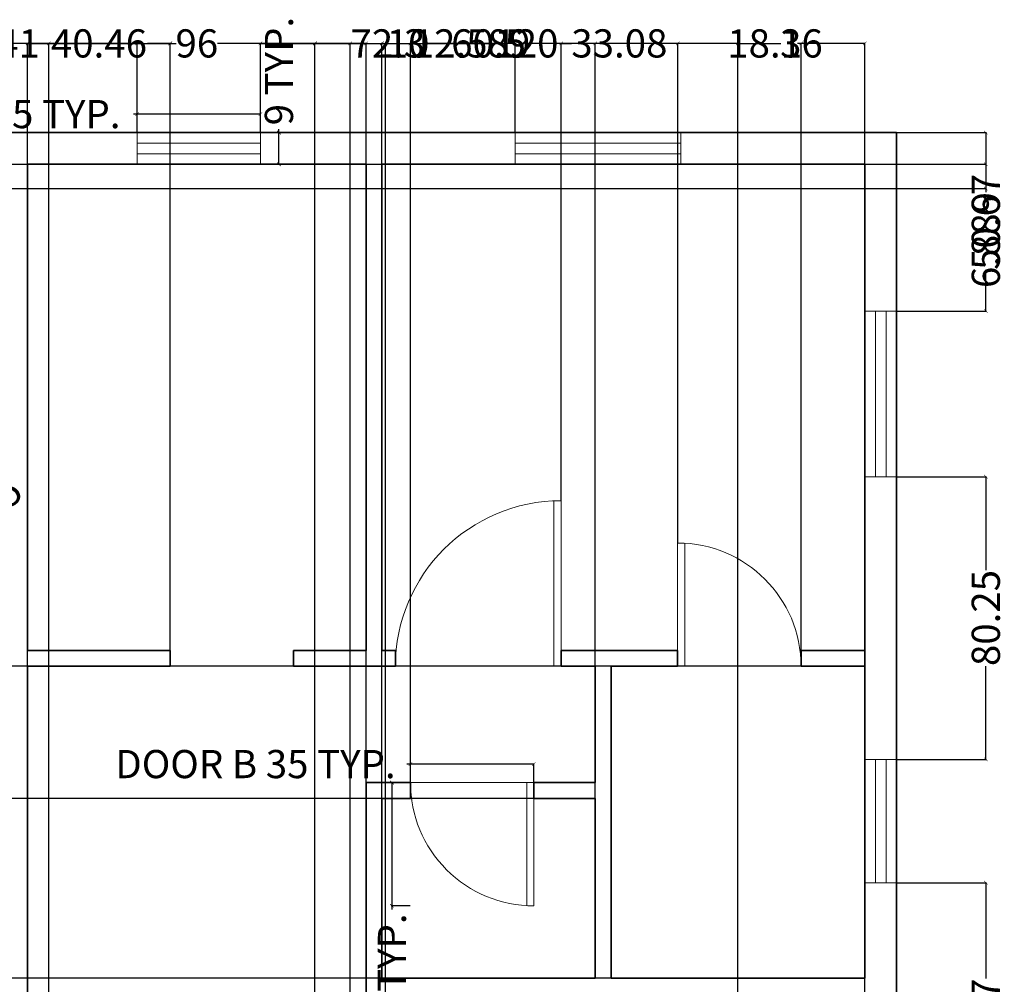
# Model space of a CAD drawing. Units: inches. Extents: x 878 to 1443, y 634 to 1188.
# Tile 5 of 5: x 1164 to 1443, y 879 to 1153. Entities that reach past the tile are written whole.
import ezdxf

# ---------------------------------------------------------------- set-up
doc = ezdxf.new("R2010")
doc.units = ezdxf.units.IN
doc.header["$MEASUREMENT"] = 0
doc.layers.add('A-ANNO-DIMS', color=2, linetype='Continuous', lineweight=18)
doc.layers.add('A-WALL', color=7, linetype='Continuous', lineweight=35)
doc.layers.add('A-DOOR', color=41, linetype='Continuous', lineweight=18, true_color=0xf4ee51)
doc.layers.add('A-GLAZ', color=152, linetype='Continuous', lineweight=18, true_color=0x2776bb)
doc.styles.get("Standard").update_dxf_attribs({"font": 'arial.ttf'})
doc.dimstyles.get("Standard").update_dxf_attribs({"dimtxt": 8, "dimasz": 1, "dimexe": 0.18, "dimexo": 0.0625, "dimgap": 0.09, "dimtad": 0, "dimdec": 4, "dimzin": 0, "dimdsep": 46, "dimlunit": 3, "dimtxsty": 'Standard', "dimblk": 'ARCHTICK', "dimcen": 0.09, "dimclrd": 6, "dimclre": 5, "dimclrt": 140, "dimadec": 0, "dimazin": 0, "dimtfac": 1, "dimtdec": 4, "dimtofl": 0, "dimtmove": 0, "dimatfit": 3, "dimfxl": 1, "dimtolj": 1, "dimtzin": 0, "dimarcsym": 0})

# ---------------------------------------------------------------- blocks, each defined once
blk = doc.blocks.new('WIN-47IN')
for p, q in [((9, 47), (0, 47)), ((0, 47), (0, 0)), ((3, 0), (3, 47)), ((6, 0), (6, 47)), ((9, 0), (9, 47)), ((0, 0), (9, 0))]:
    blk.add_line(p, q)
blk = doc.blocks.new('WIN-35IN')
for p, q in [((0, 35), (0, 0)), ((9, 35), (0, 35)), ((3, 0), (3, 35)), ((6, 0), (6, 35)), ((9, 0), (9, 35)), ((0, 0), (9, 0))]:
    blk.add_line(p, q)
blk = doc.blocks.new('DOOR-47IN')
for p, q in [((0, 47), (0, 0)), ((0, 2), (46.96, 2)), ((0, 0), (47, 0))]:
    blk.add_line(p, q)
blk.add_arc((0, 0), 47, 0, 90)
blk = doc.blocks.new('DOOR-35IN')
for p, q in [((0, 35), (0, 0)), ((2, 34.94), (2, 0)), ((0, 0), (35, 0))]:
    blk.add_line(p, q)
blk.add_arc((0, 0), 35, 360, 90)
blk = doc.blocks.new('_ArchTick')
at = {"color": 0, "linetype": 'ByBlock', "const_width": 0.15}
blk.add_lwpolyline([(-0.5, -0.5), (0.5, 0.5)], dxfattribs=at)
blk = doc.blocks.new('*D11')
at = {"layer": 'A-ANNO-DIMS', "color": 6, "lineweight": -2, "transparency": 16777216}
for p, q in [((1197.44, 1125.72), (1196.44, 1125.72)), ((1232.44, 1125.72), (1197.44, 1125.72))]:
    blk.add_line(p, q, dxfattribs=at)
at = {"layer": 'A-ANNO-DIMS', "color": 5, "lineweight": -2, "transparency": 16777216}
for p, q in [((1197.44, 1120.53), (1197.44, 1125.9)), ((1232.44, 1120.53), (1232.44, 1125.9))]:
    blk.add_line(p, q, dxfattribs=at)
at = {"layer": 'Defpoints', "color": 0, "lineweight": -2, "transparency": 16777216}
for p in [(1197.44, 1125.72), (1197.44, 1120.47), (1232.44, 1120.47)]:
    blk.add_point(p, dxfattribs=at)
at = {"layer": 'A-ANNO-DIMS', "color": 6, "lineweight": -2, "transparency": 16777216}
for p, rotation in [((1197.44, 1125.72), 179.9999999999992), ((1232.44, 1125.72), 359.9999999999992)]:
    blk.add_blockref('_ArchTick', p, dxfattribs=dict(at, rotation=rotation))
at = {"layer": 'A-ANNO-DIMS', "color": 140, "transparency": 16777216, "insert": (1145.37, 1125.72), "char_height": 8, "attachment_point": 5}
blk.add_mtext('\\A1;WINDOW B 35 TYP.', dxfattribs=at)
blk = doc.blocks.new('*D12')
at = {"layer": 'A-ANNO-DIMS', "color": 5, "lineweight": -2, "transparency": 16777216}
for p, q in [((1232.5, 1120.47), (1237.87, 1120.47)), ((1232.5, 1111.47), (1237.87, 1111.47))]:
    blk.add_line(p, q, dxfattribs=at)
at = {"layer": 'A-ANNO-DIMS', "color": 6, "lineweight": -2, "transparency": 16777216}
for p, q in [((1237.69, 1120.47), (1237.69, 1121.47)), ((1237.69, 1111.47), (1237.69, 1120.47))]:
    blk.add_line(p, q, dxfattribs=at)
at = {"layer": 'Defpoints', "color": 0, "lineweight": -2, "transparency": 16777216}
for p in [(1232.44, 1120.47), (1237.69, 1120.47), (1232.44, 1111.47)]:
    blk.add_point(p, dxfattribs=at)
at = {"layer": 'A-ANNO-DIMS', "color": 6, "lineweight": -2, "transparency": 16777216}
for p, rotation in [((1237.69, 1120.47), 90), ((1237.69, 1111.47), 270)]:
    blk.add_blockref('_ArchTick', p, dxfattribs=dict(at, rotation=rotation))
at = {"layer": 'A-ANNO-DIMS', "color": 140, "transparency": 16777216, "insert": (1237.69, 1137.92), "char_height": 8, "attachment_point": 5, "rotation": 90}
blk.add_mtext('\\A1;9 TYP.', dxfattribs=at)
blk = doc.blocks.new('*D17')
at = {"layer": 'A-ANNO-DIMS', "color": 5, "lineweight": -2, "transparency": 16777216}
for p, q in [((1274.99, 936.03), (1274.99, 941.4)), ((1309.99, 936.03), (1309.99, 941.4))]:
    blk.add_line(p, q, dxfattribs=at)
at = {"layer": 'A-ANNO-DIMS', "color": 6, "lineweight": -2, "transparency": 16777216}
for p, q in [((1274.99, 941.22), (1273.99, 941.22)), ((1309.99, 941.22), (1274.99, 941.22))]:
    blk.add_line(p, q, dxfattribs=at)
at = {"layer": 'Defpoints', "color": 0, "lineweight": -2, "transparency": 16777216}
for p in [(1274.99, 941.22), (1274.99, 935.97), (1309.99, 935.97)]:
    blk.add_point(p, dxfattribs=at)
at = {"layer": 'A-ANNO-DIMS', "color": 6, "lineweight": -2, "transparency": 16777216, "rotation": 180}
blk.add_blockref('_ArchTick', (1274.99, 941.22), dxfattribs=at)
at = {"layer": 'A-ANNO-DIMS', "color": 6, "lineweight": -2, "transparency": 16777216}
blk.add_blockref('_ArchTick', (1309.99, 941.22), dxfattribs=at)
at = {"layer": 'A-ANNO-DIMS', "color": 140, "transparency": 16777216, "insert": (1231.03, 941.22), "char_height": 8, "attachment_point": 5}
blk.add_mtext('\\A1;DOOR B 35 TYP.', dxfattribs=at)
blk = doc.blocks.new('*D18')
at = {"layer": 'A-ANNO-DIMS', "color": 5, "lineweight": -2, "transparency": 16777216}
for p, q in [((1274.92, 935.97), (1269.56, 935.97)), ((1274.92, 900.97), (1269.56, 900.97))]:
    blk.add_line(p, q, dxfattribs=at)
at = {"layer": 'A-ANNO-DIMS', "color": 6, "lineweight": -2, "transparency": 16777216}
for p, q in [((1269.74, 935.97), (1269.74, 900.97)), ((1269.74, 900.97), (1269.74, 899.97))]:
    blk.add_line(p, q, dxfattribs=at)
at = {"layer": 'Defpoints', "color": 0, "lineweight": -2, "transparency": 16777216}
for p in [(1274.99, 935.97), (1269.74, 900.97), (1274.99, 900.97)]:
    blk.add_point(p, dxfattribs=at)
at = {"layer": 'A-ANNO-DIMS', "color": 6, "lineweight": -2, "transparency": 16777216}
for p, rotation in [((1269.74, 935.97), 90), ((1269.74, 900.97), 270)]:
    blk.add_blockref('_ArchTick', p, dxfattribs=dict(at, rotation=rotation))
at = {"layer": 'A-ANNO-DIMS', "color": 140, "transparency": 16777216, "insert": (1269.74, 880.41), "char_height": 8, "attachment_point": 5, "rotation": 90}
blk.add_mtext('\\A1;35 TYP.', dxfattribs=at)
blk = doc.blocks.new('*D26')
at = {"layer": 'A-ANNO-DIMS', "color": 5, "lineweight": -2, "transparency": 16777216}
for p, q in [((1115.03, 1120.53), (1115.03, 1145.96)), ((1197.44, 1120.53), (1197.44, 1145.96))]:
    blk.add_line(p, q, dxfattribs=at)
at = {"layer": 'A-ANNO-DIMS', "color": 6, "lineweight": -2, "transparency": 16777216}
for p, q in [((1115.03, 1145.78), (1143.42, 1145.78)), ((1197.44, 1145.78), (1169.06, 1145.78))]:
    blk.add_line(p, q, dxfattribs=at)
at = {"layer": 'Defpoints', "color": 0, "lineweight": -2, "transparency": 16777216}
for p in [(1197.44, 1145.78), (1115.03, 1120.47), (1197.44, 1120.47)]:
    blk.add_point(p, dxfattribs=at)
at = {"layer": 'A-ANNO-DIMS', "color": 6, "lineweight": -2, "transparency": 16777216, "rotation": 180}
blk.add_blockref('_ArchTick', (1115.03, 1145.78), dxfattribs=at)
at = {"layer": 'A-ANNO-DIMS', "color": 6, "lineweight": -2, "transparency": 16777216}
blk.add_blockref('_ArchTick', (1197.44, 1145.78), dxfattribs=at)
at = {"layer": 'A-ANNO-DIMS', "color": 140, "transparency": 16777216, "insert": (1156.24, 1145.78), "char_height": 8, "attachment_point": 5}
blk.add_mtext('\\A1;82.41', dxfattribs=at)
blk = doc.blocks.new('*D27')
at = {"layer": 'A-ANNO-DIMS', "color": 5, "lineweight": -2, "transparency": 16777216}
for p, q in [((1232.44, 1120.53), (1232.44, 1145.96)), ((1304.74, 1120.53), (1304.74, 1145.96))]:
    blk.add_line(p, q, dxfattribs=at)
at = {"layer": 'A-ANNO-DIMS', "color": 6, "lineweight": -2, "transparency": 16777216}
for p, q in [((1232.44, 1145.78), (1258.14, 1145.78)), ((1304.74, 1145.78), (1279.04, 1145.78))]:
    blk.add_line(p, q, dxfattribs=at)
at = {"layer": 'Defpoints', "color": 0, "lineweight": -2, "transparency": 16777216}
for p in [(1304.74, 1145.78), (1232.44, 1120.47), (1304.74, 1120.47)]:
    blk.add_point(p, dxfattribs=at)
at = {"layer": 'A-ANNO-DIMS', "color": 6, "lineweight": -2, "transparency": 16777216, "rotation": 180}
blk.add_blockref('_ArchTick', (1232.44, 1145.78), dxfattribs=at)
at = {"layer": 'A-ANNO-DIMS', "color": 6, "lineweight": -2, "transparency": 16777216}
blk.add_blockref('_ArchTick', (1304.74, 1145.78), dxfattribs=at)
at = {"layer": 'A-ANNO-DIMS', "color": 140, "transparency": 16777216, "insert": (1268.59, 1145.78), "char_height": 8, "attachment_point": 5}
blk.add_mtext('\\A1;72.3', dxfattribs=at)
blk = doc.blocks.new('*D30')
at = {"layer": 'A-ANNO-DIMS', "color": 5, "lineweight": -2, "transparency": 16777216}
for p, q in [((1412.96, 1120.47), (1438.39, 1120.47)), ((1412.96, 1069.8), (1438.39, 1069.8))]:
    blk.add_line(p, q, dxfattribs=at)
at = {"layer": 'A-ANNO-DIMS', "color": 6, "lineweight": -2, "transparency": 16777216}
for p, q in [((1438.21, 1120.47), (1438.21, 1108.72)), ((1438.21, 1069.8), (1438.21, 1081.55))]:
    blk.add_line(p, q, dxfattribs=at)
at = {"layer": 'Defpoints', "color": 0, "lineweight": -2, "transparency": 16777216}
for p in [(1412.9, 1120.47), (1412.9, 1069.8), (1438.21, 1069.8)]:
    blk.add_point(p, dxfattribs=at)
at = {"layer": 'A-ANNO-DIMS', "color": 6, "lineweight": -2, "transparency": 16777216}
for p, rotation in [((1438.21, 1120.47), 90), ((1438.21, 1069.8), 270)]:
    blk.add_blockref('_ArchTick', p, dxfattribs=dict(at, rotation=rotation))
at = {"layer": 'A-ANNO-DIMS', "color": 140, "transparency": 16777216, "insert": (1438.21, 1095.14), "char_height": 8, "attachment_point": 5, "rotation": 90}
blk.add_mtext('\\A1;50.67', dxfattribs=at)
blk = doc.blocks.new('*D31')
at = {"layer": 'A-ANNO-DIMS', "color": 5, "lineweight": -2, "transparency": 16777216}
for p, q in [((1412.96, 1022.8), (1438.39, 1022.8)), ((1412.96, 942.55), (1438.39, 942.55))]:
    blk.add_line(p, q, dxfattribs=at)
at = {"layer": 'A-ANNO-DIMS', "color": 6, "lineweight": -2, "transparency": 16777216}
for p, q in [((1438.21, 1022.8), (1438.21, 996.3)), ((1438.21, 942.55), (1438.21, 969.05))]:
    blk.add_line(p, q, dxfattribs=at)
at = {"layer": 'Defpoints', "color": 0, "lineweight": -2, "transparency": 16777216}
for p in [(1412.9, 1022.8), (1412.9, 942.55), (1438.21, 942.55)]:
    blk.add_point(p, dxfattribs=at)
at = {"layer": 'A-ANNO-DIMS', "color": 6, "lineweight": -2, "transparency": 16777216}
for p, rotation in [((1438.21, 1022.8), 90), ((1438.21, 942.55), 270)]:
    blk.add_blockref('_ArchTick', p, dxfattribs=dict(at, rotation=rotation))
at = {"layer": 'A-ANNO-DIMS', "color": 140, "transparency": 16777216, "insert": (1438.21, 982.68), "char_height": 8, "attachment_point": 5, "rotation": 90}
blk.add_mtext('\\A1;80.25', dxfattribs=at)
blk = doc.blocks.new('*D32')
at = {"layer": 'A-ANNO-DIMS', "color": 5, "lineweight": -2, "transparency": 16777216}
for p, q in [((1412.96, 907.55), (1438.39, 907.55)), ((1412.96, 825.89), (1438.39, 825.89))]:
    blk.add_line(p, q, dxfattribs=at)
at = {"layer": 'A-ANNO-DIMS', "color": 6, "lineweight": -2, "transparency": 16777216}
for p, q in [((1438.21, 907.55), (1438.21, 880.32)), ((1438.21, 825.89), (1438.21, 853.13))]:
    blk.add_line(p, q, dxfattribs=at)
at = {"layer": 'Defpoints', "color": 0, "lineweight": -2, "transparency": 16777216}
for p in [(1412.9, 907.55), (1412.9, 825.89), (1438.21, 825.89)]:
    blk.add_point(p, dxfattribs=at)
at = {"layer": 'A-ANNO-DIMS', "color": 6, "lineweight": -2, "transparency": 16777216}
for p, rotation in [((1438.21, 907.55), 90), ((1438.21, 825.89), 270)]:
    blk.add_blockref('_ArchTick', p, dxfattribs=dict(at, rotation=rotation))
at = {"layer": 'A-ANNO-DIMS', "color": 140, "transparency": 16777216, "insert": (1438.21, 866.72), "char_height": 8, "attachment_point": 5, "rotation": 90}
blk.add_mtext('\\A1;81.67', dxfattribs=at)
blk = doc.blocks.new('*D35')
at = {"layer": 'A-ANNO-DIMS', "color": 5, "lineweight": -2, "transparency": 16777216}
for p, q in [((1166.4, 760.53), (1166.4, 1145.96)), ((1262.4, 760.53), (1262.4, 1145.96))]:
    blk.add_line(p, q, dxfattribs=at)
at = {"layer": 'A-ANNO-DIMS', "color": 6, "lineweight": -2, "transparency": 16777216}
for p, q in [((1166.4, 1145.78), (1208.58, 1145.78)), ((1262.4, 1145.78), (1220.22, 1145.78))]:
    blk.add_line(p, q, dxfattribs=at)
at = {"layer": 'Defpoints', "color": 0, "lineweight": -2, "transparency": 16777216}
for p in [(1262.4, 1145.78), (1166.4, 760.47), (1262.4, 760.47)]:
    blk.add_point(p, dxfattribs=at)
at = {"layer": 'A-ANNO-DIMS', "color": 6, "lineweight": -2, "transparency": 16777216, "rotation": 180}
blk.add_blockref('_ArchTick', (1166.4, 1145.78), dxfattribs=at)
at = {"layer": 'A-ANNO-DIMS', "color": 6, "lineweight": -2, "transparency": 16777216}
blk.add_blockref('_ArchTick', (1262.4, 1145.78), dxfattribs=at)
at = {"layer": 'A-ANNO-DIMS', "color": 140, "transparency": 16777216, "insert": (1214.4, 1145.78), "char_height": 8, "attachment_point": 5}
blk.add_mtext('\\A1;96', dxfattribs=at)
blk = doc.blocks.new('*D37')
at = {"layer": 'A-ANNO-DIMS', "color": 5, "lineweight": -2, "transparency": 16777216}
for p, q in [((1403.84, 968.97), (883.41, 968.97)), ((1403.84, 880.47), (883.41, 880.47))]:
    blk.add_line(p, q, dxfattribs=at)
at = {"layer": 'A-ANNO-DIMS', "color": 6, "lineweight": -2, "transparency": 16777216}
for p, q in [((883.59, 968.97), (883.59, 935.24)), ((883.59, 880.47), (883.59, 914.2))]:
    blk.add_line(p, q, dxfattribs=at)
at = {"layer": 'Defpoints', "color": 0, "lineweight": -2, "transparency": 16777216}
for p in [(1403.9, 968.97), (883.59, 880.47), (1403.9, 880.47)]:
    blk.add_point(p, dxfattribs=at)
at = {"layer": 'A-ANNO-DIMS', "color": 6, "lineweight": -2, "transparency": 16777216}
for p, rotation in [((883.59, 968.97), 90), ((883.59, 880.47), 270)]:
    blk.add_blockref('_ArchTick', p, dxfattribs=dict(at, rotation=rotation))
at = {"layer": 'A-ANNO-DIMS', "color": 140, "transparency": 16777216, "insert": (883.59, 924.72), "char_height": 8, "attachment_point": 5, "rotation": 90}
blk.add_mtext('\\A1;88.5', dxfattribs=at)
blk = doc.blocks.new('*D41')
at = {"layer": 'A-ANNO-DIMS', "color": 5, "lineweight": -2, "transparency": 16777216}
for p, q in [((1266.9, 880.53), (1266.9, 1145.96)), ((1327.4, 880.53), (1327.4, 1145.96))]:
    blk.add_line(p, q, dxfattribs=at)
at = {"layer": 'A-ANNO-DIMS', "color": 6, "lineweight": -2, "transparency": 16777216}
for p, q in [((1266.9, 1145.78), (1286.62, 1145.78)), ((1327.4, 1145.78), (1307.68, 1145.78))]:
    blk.add_line(p, q, dxfattribs=at)
at = {"layer": 'Defpoints', "color": 0, "lineweight": -2, "transparency": 16777216}
for p in [(1327.4, 1145.78), (1266.9, 880.47), (1327.4, 880.47)]:
    blk.add_point(p, dxfattribs=at)
at = {"layer": 'A-ANNO-DIMS', "color": 6, "lineweight": -2, "transparency": 16777216, "rotation": 180}
blk.add_blockref('_ArchTick', (1266.9, 1145.78), dxfattribs=at)
at = {"layer": 'A-ANNO-DIMS', "color": 6, "lineweight": -2, "transparency": 16777216}
blk.add_blockref('_ArchTick', (1327.4, 1145.78), dxfattribs=at)
at = {"layer": 'A-ANNO-DIMS', "color": 140, "transparency": 16777216, "insert": (1297.15, 1145.78), "char_height": 8, "attachment_point": 5}
blk.add_mtext('\\A1;60.5', dxfattribs=at)
blk = doc.blocks.new('*D43')
at = {"layer": 'A-ANNO-DIMS', "color": 5, "lineweight": -2, "transparency": 16777216}
for p, q in [((1327.34, 931.47), (883.41, 931.47)), ((1327.34, 880.47), (883.41, 880.47))]:
    blk.add_line(p, q, dxfattribs=at)
at = {"layer": 'A-ANNO-DIMS', "color": 6, "lineweight": -2, "transparency": 16777216}
for p, q in [((883.59, 931.47), (883.59, 911.02)), ((883.59, 880.47), (883.59, 900.92))]:
    blk.add_line(p, q, dxfattribs=at)
at = {"layer": 'Defpoints', "color": 0, "lineweight": -2, "transparency": 16777216}
for p in [(883.59, 931.47), (1327.4, 931.47), (1327.4, 880.47)]:
    blk.add_point(p, dxfattribs=at)
at = {"layer": 'A-ANNO-DIMS', "color": 6, "lineweight": -2, "transparency": 16777216}
for p, rotation in [((883.59, 931.47), 90), ((883.59, 880.47), 270)]:
    blk.add_blockref('_ArchTick', p, dxfattribs=dict(at, rotation=rotation))
at = {"layer": 'A-ANNO-DIMS', "color": 140, "transparency": 16777216, "insert": (883.59, 905.97), "char_height": 8, "attachment_point": 5, "rotation": 90}
blk.add_mtext('\\A1;51', dxfattribs=at)
blk = doc.blocks.new('*D46')
at = {"layer": 'A-ANNO-DIMS', "color": 5, "lineweight": -2, "transparency": 16777216}
for p, q in [((1110.3, 751.53), (1110.3, 1145.96)), ((1172.39, 751.53), (1172.39, 1145.96))]:
    blk.add_line(p, q, dxfattribs=at)
at = {"layer": 'A-ANNO-DIMS', "color": 6, "lineweight": -2, "transparency": 16777216}
for p, q in [((1110.3, 1145.78), (1127.73, 1145.78)), ((1172.39, 1145.78), (1154.96, 1145.78))]:
    blk.add_line(p, q, dxfattribs=at)
at = {"layer": 'Defpoints', "color": 0, "lineweight": -2, "transparency": 16777216}
for p in [(1172.39, 1145.78), (1110.3, 751.47), (1172.39, 751.47)]:
    blk.add_point(p, dxfattribs=at)
at = {"layer": 'A-ANNO-DIMS', "color": 6, "lineweight": -2, "transparency": 16777216, "rotation": 180}
blk.add_blockref('_ArchTick', (1110.3, 1145.78), dxfattribs=at)
at = {"layer": 'A-ANNO-DIMS', "color": 6, "lineweight": -2, "transparency": 16777216}
blk.add_blockref('_ArchTick', (1172.39, 1145.78), dxfattribs=at)
at = {"layer": 'A-ANNO-DIMS', "color": 140, "transparency": 16777216, "insert": (1141.35, 1145.78), "char_height": 8, "attachment_point": 5}
blk.add_mtext('\\A1;62.08', dxfattribs=at)
blk = doc.blocks.new('*D51')
at = {"layer": 'A-ANNO-DIMS', "color": 5, "lineweight": -2, "transparency": 16777216}
for p, q in [((1166.4, 973.53), (1166.4, 1145.96)), ((1206.86, 973.53), (1206.86, 1145.96))]:
    blk.add_line(p, q, dxfattribs=at)
at = {"layer": 'A-ANNO-DIMS', "color": 6, "lineweight": -2, "transparency": 16777216}
for p, q in [((1166.4, 1145.78), (1172.88, 1145.78)), ((1206.86, 1145.78), (1200.37, 1145.78))]:
    blk.add_line(p, q, dxfattribs=at)
at = {"layer": 'Defpoints', "color": 0, "lineweight": -2, "transparency": 16777216}
for p in [(1206.86, 1145.78), (1166.4, 973.47), (1206.86, 973.47)]:
    blk.add_point(p, dxfattribs=at)
at = {"layer": 'A-ANNO-DIMS', "color": 6, "lineweight": -2, "transparency": 16777216, "rotation": 180}
blk.add_blockref('_ArchTick', (1166.4, 1145.78), dxfattribs=at)
at = {"layer": 'A-ANNO-DIMS', "color": 6, "lineweight": -2, "transparency": 16777216}
blk.add_blockref('_ArchTick', (1206.86, 1145.78), dxfattribs=at)
at = {"layer": 'A-ANNO-DIMS', "color": 140, "transparency": 16777216, "insert": (1186.63, 1145.78), "char_height": 8, "attachment_point": 5}
blk.add_mtext('\\A1;40.46', dxfattribs=at)
blk = doc.blocks.new('*D54')
at = {"layer": 'A-ANNO-DIMS', "color": 6, "lineweight": -2, "transparency": 16777216}
for p, q in [((1385.8, 1145.78), (1384.8, 1145.78)), ((1403.9, 1145.78), (1385.8, 1145.78))]:
    blk.add_line(p, q, dxfattribs=at)
at = {"layer": 'A-ANNO-DIMS', "color": 5, "lineweight": -2, "transparency": 16777216}
for p, q in [((1385.8, 973.53), (1385.8, 1145.96)), ((1403.9, 973.53), (1403.9, 1145.96))]:
    blk.add_line(p, q, dxfattribs=at)
at = {"layer": 'Defpoints', "color": 0, "lineweight": -2, "transparency": 16777216}
for p in [(1385.8, 1145.78), (1385.8, 973.47), (1403.9, 973.47)]:
    blk.add_point(p, dxfattribs=at)
at = {"layer": 'A-ANNO-DIMS', "color": 6, "lineweight": -2, "transparency": 16777216, "rotation": 180}
blk.add_blockref('_ArchTick', (1385.8, 1145.78), dxfattribs=at)
at = {"layer": 'A-ANNO-DIMS', "color": 6, "lineweight": -2, "transparency": 16777216}
blk.add_blockref('_ArchTick', (1403.9, 1145.78), dxfattribs=at)
at = {"layer": 'A-ANNO-DIMS', "color": 140, "transparency": 16777216, "insert": (1375.47, 1145.78), "char_height": 8, "attachment_point": 5}
blk.add_mtext('\\A1;18.1', dxfattribs=at)
blk = doc.blocks.new('*D55')
at = {"layer": 'A-ANNO-DIMS', "color": 5, "lineweight": -2, "transparency": 16777216}
for p, q in [((1317.72, 1016.03), (1317.72, 1145.96)), ((1350.8, 1004.03), (1350.8, 1145.96))]:
    blk.add_line(p, q, dxfattribs=at)
at = {"layer": 'A-ANNO-DIMS', "color": 6, "lineweight": -2, "transparency": 16777216}
for p, q in [((1317.72, 1145.78), (1320.66, 1145.78)), ((1350.8, 1145.78), (1347.85, 1145.78))]:
    blk.add_line(p, q, dxfattribs=at)
at = {"layer": 'Defpoints', "color": 0, "lineweight": -2, "transparency": 16777216}
for p in [(1350.8, 1145.78), (1317.72, 1015.97), (1350.8, 1003.97)]:
    blk.add_point(p, dxfattribs=at)
at = {"layer": 'A-ANNO-DIMS', "color": 6, "lineweight": -2, "transparency": 16777216, "rotation": 180}
blk.add_blockref('_ArchTick', (1317.72, 1145.78), dxfattribs=at)
at = {"layer": 'A-ANNO-DIMS', "color": 6, "lineweight": -2, "transparency": 16777216}
blk.add_blockref('_ArchTick', (1350.8, 1145.78), dxfattribs=at)
at = {"layer": 'A-ANNO-DIMS', "color": 140, "transparency": 16777216, "insert": (1334.26, 1145.78), "char_height": 8, "attachment_point": 5}
blk.add_mtext('\\A1;33.08', dxfattribs=at)
blk = doc.blocks.new('*D57')
at = {"layer": 'A-ANNO-DIMS', "color": 5, "lineweight": -2, "transparency": 16777216}
for p, q in [((1262.4, 936.03), (1262.4, 1145.96)), ((1274.99, 936.03), (1274.99, 1145.96))]:
    blk.add_line(p, q, dxfattribs=at)
at = {"layer": 'A-ANNO-DIMS', "color": 6, "lineweight": -2, "transparency": 16777216}
for p, q in [((1262.4, 1145.78), (1274.99, 1145.78)), ((1274.99, 1145.78), (1275.99, 1145.78))]:
    blk.add_line(p, q, dxfattribs=at)
at = {"layer": 'Defpoints', "color": 0, "lineweight": -2, "transparency": 16777216}
for p in [(1274.99, 1145.78), (1262.4, 935.97), (1274.99, 935.97)]:
    blk.add_point(p, dxfattribs=at)
at = {"layer": 'A-ANNO-DIMS', "color": 6, "lineweight": -2, "transparency": 16777216, "rotation": 180}
blk.add_blockref('_ArchTick', (1262.4, 1145.78), dxfattribs=at)
at = {"layer": 'A-ANNO-DIMS', "color": 6, "lineweight": -2, "transparency": 16777216}
blk.add_blockref('_ArchTick', (1274.99, 1145.78), dxfattribs=at)
at = {"layer": 'A-ANNO-DIMS', "color": 140, "transparency": 16777216, "insert": (1292.31, 1145.78), "char_height": 8, "attachment_point": 5}
blk.add_mtext('\\A1;12.589', dxfattribs=at)
blk = doc.blocks.new('*D58')
at = {"layer": 'A-ANNO-DIMS', "color": 5, "lineweight": -2, "transparency": 16777216}
for p, q in [((1367.9, 673.53), (1367.9, 1145.96)), ((1403.9, 673.53), (1403.9, 1145.96))]:
    blk.add_line(p, q, dxfattribs=at)
at = {"layer": 'A-ANNO-DIMS', "color": 6, "lineweight": -2, "transparency": 16777216}
for p, q in [((1367.9, 1145.78), (1380.08, 1145.78)), ((1403.9, 1145.78), (1391.71, 1145.78))]:
    blk.add_line(p, q, dxfattribs=at)
at = {"layer": 'Defpoints', "color": 0, "lineweight": -2, "transparency": 16777216}
for p in [(1403.9, 1145.78), (1367.9, 673.47), (1403.9, 673.47)]:
    blk.add_point(p, dxfattribs=at)
at = {"layer": 'A-ANNO-DIMS', "color": 6, "lineweight": -2, "transparency": 16777216, "rotation": 180}
blk.add_blockref('_ArchTick', (1367.9, 1145.78), dxfattribs=at)
at = {"layer": 'A-ANNO-DIMS', "color": 6, "lineweight": -2, "transparency": 16777216}
blk.add_blockref('_ArchTick', (1403.9, 1145.78), dxfattribs=at)
at = {"layer": 'A-ANNO-DIMS', "color": 140, "transparency": 16777216, "insert": (1385.9, 1145.78), "char_height": 8, "attachment_point": 5}
blk.add_mtext('\\A1;36', dxfattribs=at)
blk = doc.blocks.new('*D59')
at = {"layer": 'A-ANNO-DIMS', "color": 5, "lineweight": -2, "transparency": 16777216}
for p, q in [((1247.9, 709.53), (1247.9, 1145.96)), ((1367.9, 709.53), (1367.9, 1145.96))]:
    blk.add_line(p, q, dxfattribs=at)
at = {"layer": 'A-ANNO-DIMS', "color": 6, "lineweight": -2, "transparency": 16777216}
for p, q in [((1247.9, 1145.78), (1299.36, 1145.78)), ((1367.9, 1145.78), (1316.44, 1145.78))]:
    blk.add_line(p, q, dxfattribs=at)
at = {"layer": 'Defpoints', "color": 0, "lineweight": -2, "transparency": 16777216}
for p in [(1367.9, 1145.78), (1247.9, 709.47), (1367.9, 709.47)]:
    blk.add_point(p, dxfattribs=at)
at = {"layer": 'A-ANNO-DIMS', "color": 6, "lineweight": -2, "transparency": 16777216, "rotation": 180}
blk.add_blockref('_ArchTick', (1247.9, 1145.78), dxfattribs=at)
at = {"layer": 'A-ANNO-DIMS', "color": 6, "lineweight": -2, "transparency": 16777216}
blk.add_blockref('_ArchTick', (1367.9, 1145.78), dxfattribs=at)
at = {"layer": 'A-ANNO-DIMS', "color": 140, "transparency": 16777216, "insert": (1307.9, 1145.78), "char_height": 8, "attachment_point": 5}
blk.add_mtext('\\A1;120', dxfattribs=at)
blk = doc.blocks.new('*D62')
at = {"layer": 'A-ANNO-DIMS', "color": 5, "lineweight": -2, "transparency": 16777216}
for p, q in [((1257.9, 751.53), (1257.9, 1145.96)), ((1267.9, 751.53), (1267.9, 1145.96))]:
    blk.add_line(p, q, dxfattribs=at)
at = {"layer": 'A-ANNO-DIMS', "color": 6, "lineweight": -2, "transparency": 16777216}
for p, q in [((1257.9, 1145.78), (1267.9, 1145.78)), ((1267.9, 1145.78), (1268.9, 1145.78))]:
    blk.add_line(p, q, dxfattribs=at)
at = {"layer": 'Defpoints', "color": 0, "lineweight": -2, "transparency": 16777216}
for p in [(1267.9, 1145.78), (1257.9, 751.47), (1267.9, 751.47)]:
    blk.add_point(p, dxfattribs=at)
at = {"layer": 'A-ANNO-DIMS', "color": 6, "lineweight": -2, "transparency": 16777216, "rotation": 180}
blk.add_blockref('_ArchTick', (1257.9, 1145.78), dxfattribs=at)
at = {"layer": 'A-ANNO-DIMS', "color": 6, "lineweight": -2, "transparency": 16777216}
blk.add_blockref('_ArchTick', (1267.9, 1145.78), dxfattribs=at)
at = {"layer": 'A-ANNO-DIMS', "color": 140, "transparency": 16777216, "insert": (1274.33, 1145.78), "char_height": 8, "attachment_point": 5}
blk.add_mtext('\\A1;10', dxfattribs=at)
blk = doc.blocks.new('*D67')
at = {"layer": 'A-ANNO-DIMS', "color": 5, "lineweight": -2, "transparency": 16777216}
for p, q in [((985.14, 1111.47), (1438.39, 1111.47)), ((983.27, 1104.58), (1438.39, 1104.58))]:
    blk.add_line(p, q, dxfattribs=at)
at = {"layer": 'A-ANNO-DIMS', "color": 6, "lineweight": -2, "transparency": 16777216}
for p, q in [((1438.21, 1111.47), (1438.21, 1104.58)), ((1438.21, 1104.58), (1438.21, 1103.58))]:
    blk.add_line(p, q, dxfattribs=at)
at = {"layer": 'Defpoints', "color": 0, "lineweight": -2, "transparency": 16777216}
for p in [(985.07, 1111.47), (983.2, 1104.58), (1438.21, 1104.58)]:
    blk.add_point(p, dxfattribs=at)
at = {"layer": 'A-ANNO-DIMS', "color": 6, "lineweight": -2, "transparency": 16777216}
for p, rotation in [((1438.21, 1111.47), 90), ((1438.21, 1104.58), 270)]:
    blk.add_blockref('_ArchTick', p, dxfattribs=dict(at, rotation=rotation))
at = {"layer": 'A-ANNO-DIMS', "color": 140, "transparency": 16777216, "insert": (1438.21, 1089.96), "char_height": 8, "attachment_point": 5, "rotation": 90}
blk.add_mtext('\\A1;6.889', dxfattribs=at)
blk = doc.blocks.new('*D70')
at = {"layer": 'A-ANNO-DIMS', "color": 6, "lineweight": -2, "transparency": 16777216}
blk.add_line((1137.88, 995.53), (1136.07, 993.72), dxfattribs=at)
at = {"layer": 'A-ANNO-DIMS', "color": 5, "lineweight": -2, "transparency": 16777216}
for p, q in [((1111.23, 968.97), (1111.41, 968.97)), ((1111.32, 968.88), (1111.32, 969.06))]:
    blk.add_line(p, q, dxfattribs=at)
at = {"layer": 'Defpoints', "color": 0, "lineweight": -2, "transparency": 16777216}
for p in [(1136.07, 993.72), (1111.32, 968.97)]:
    blk.add_point(p, dxfattribs=at)
at = {"layer": 'A-ANNO-DIMS', "color": 6, "lineweight": -2, "transparency": 16777216, "rotation": 224.9999525404688}
blk.add_blockref('_ArchTick', (1136.07, 993.72), dxfattribs=at)
at = {"layer": 'A-ANNO-DIMS', "color": 140, "transparency": 16777216, "insert": (1150.92, 1008.57), "char_height": 8, "attachment_point": 5, "rotation": 45}
blk.add_mtext('\\A1;4X R35', dxfattribs=at)

msp = doc.modelspace()

# ---------------------------------------------------------------- linework, layer by layer
at = {"layer": 'A-WALL'}
for p, q in [((908.8987, 1120.4702), (1412.8987, 1120.4702)), ((1412.8987, 1120.4702), (1412.8987, 664.4702)), ((1166.3987, 1111.4702), (1166.3987, 973.4702)), ((1166.3987, 1111.4702), (1262.3987, 1111.4702)), ((1262.3987, 1111.4702), (1262.3987, 973.4702)), ((1266.8987, 1111.4702), (1266.8987, 973.4702)), ((1266.8987, 1111.4702), (1403.8987, 1111.4702)), ((1403.8987, 1111.4702), (1403.8987, 880.4702)), ((1206.8579, 973.4702), (1166.3987, 973.4702)), ((1206.8579, 968.9702), (1206.8579, 973.4702)), ((1262.3987, 973.4702), (1241.8579, 973.4702)), ((1241.8579, 968.9702), (1241.8579, 973.4702)), ((1270.7151, 973.4702), (1266.8987, 973.4702)), ((1270.7151, 968.9702), (1270.7151, 973.4702)), ((1350.7981, 973.4702), (1317.7151, 973.4702)), ((1317.7151, 968.9702), (1317.7151, 973.4702)), ((1350.7981, 973.4702), (1350.7981, 968.9702)), ((1403.8987, 973.4702), (1385.7981, 973.4702)), ((1385.7981, 973.4702), (1385.7981, 968.9702)), ((1166.3987, 968.9702), (1166.3987, 760.4702)), ((1206.8579, 968.9702), (1166.3987, 968.9702)), ((1270.7151, 968.9702), (1241.8579, 968.9702)), ((1327.3987, 968.9702), (1317.7151, 968.9702)), ((1327.3987, 968.9702), (1327.3987, 935.9702)), ((1331.8987, 968.9702), (1331.8987, 880.4702)), ((1350.7981, 968.9702), (1331.8987, 968.9702)), ((1403.8987, 968.9702), (1385.7981, 968.9702)), ((1262.3987, 935.9702), (1262.3987, 856.1495)), ((1274.9872, 935.9702), (1262.3987, 935.9702)), ((1274.9872, 931.4702), (1274.9872, 935.9702)), ((1327.3987, 935.9702), (1309.9872, 935.9702)), ((1309.9872, 931.4702), (1309.9872, 935.9702)), ((1266.8987, 931.4702), (1266.8987, 880.4702)), ((1274.9872, 931.4702), (1266.8987, 931.4702)), ((1327.3987, 931.4702), (1309.9872, 931.4702)), ((1327.3987, 931.4702), (1327.3987, 880.4702)), ((1327.3987, 880.4702), (1266.8987, 880.4702)), ((1403.8987, 880.4702), (1331.8987, 880.4702))]:
    msp.add_line(p, q, dxfattribs=at)

# ---------------------------------------------------------------- block references
at = {"layer": 'A-DOOR'}
for name, p, rotation in [('DOOR-47IN', (1317.7151, 968.9702), 90.00000000000036), ('DOOR-35IN', (1309.9872, 935.9702), 180)]:
    msp.add_blockref(name, p, dxfattribs=dict(at, rotation=rotation))
msp.add_blockref('DOOR-35IN', (1350.7981, 968.9702), dxfattribs=at)
at = {"layer": 'A-GLAZ'}
for name, p, rotation in [('WIN-35IN', (1232.4415, 1111.4702), 89.9999999999994), ('WIN-47IN', (1304.7374, 1120.4702), 269.9999999999993)]:
    msp.add_blockref(name, p, dxfattribs=dict(at, rotation=rotation))
for name, p in [('WIN-47IN', (1403.8987, 1022.8001)), ('WIN-35IN', (1403.8987, 907.5545))]:
    msp.add_blockref(name, p, dxfattribs=at)

# ---------------------------------------------------------------- dimensions: what is measured, and where the dimension line sits
at = {"layer": 'A-ANNO-DIMS'}
for base, p1, p2, angle, text, picture, middle in [((1197.4415, 1125.7202), (1232.4415, 1120.4702), (1197.4415, 1120.4702), 180, 'WINDOW B <> TYP.', '*D11', (1145.3665, 1125.7202)), ((1237.6915, 1120.4702), (1232.4415, 1111.4702), (1232.4415, 1120.4702), 90, '<> TYP.', '*D12', (1237.6915, 1137.9231)), ((1274.9872, 941.2202), (1309.9872, 935.9702), (1274.9872, 935.9702), 180, 'DOOR B <> TYP.', '*D17', (1231.0295, 941.2202)), ((1269.7372, 900.9702), (1274.9872, 935.9702), (1274.9872, 900.9702), 270, '<> TYP.', '*D18', (1269.7372, 880.4123))]:
    dim = msp.add_linear_dim(base=base, p1=p1, p2=p2, angle=angle, text=text, dimstyle='Standard', override={"dimdec": 0, "dimlfac": 1, "dimrnd": 0, "dimzin": 0, "dimdsep": 46, "dimlunit": 2}, dxfattribs=at)
    dim.commit()
    dim.dimension.update_dxf_attribs({"geometry": picture, "text_midpoint": middle})
for base, p1, p2, override, picture, middle in [((1172.3876, 1145.7802), (1110.3038, 751.4702), (1172.3876, 751.4702), {"dimdec": 2, "dimlfac": 1, "dimrnd": 0, "dimzin": 0, "dimdsep": 46, "dimlunit": 2}, '*D46', (1141.3457, 1145.7802)), ((1197.4415, 1145.7802), (1115.0314, 1120.4702), (1197.4415, 1120.4702), {"dimdec": 2, "dimlfac": 1, "dimrnd": 0, "dimzin": 0, "dimdsep": 46, "dimlunit": 2}, '*D26', (1156.2364, 1145.7802)), ((1262.3987, 1145.7802), (1166.3987, 760.4702), (1262.3987, 760.4702), {"dimdec": 0, "dimlfac": 1, "dimrnd": 0, "dimzin": 0, "dimdsep": 46, "dimlunit": 2}, '*D35', (1214.3987, 1145.7802)), ((1206.8579, 1145.7802), (1166.3987, 973.4702), (1206.8579, 973.4702), {"dimdec": 2, "dimlfac": 1, "dimrnd": 0, "dimzin": 0, "dimdsep": 46, "dimlunit": 2}, '*D51', (1186.6283, 1145.7802)), ((1304.7374, 1145.7802), (1232.4415, 1120.4702), (1304.7374, 1120.4702), {"dimdec": 1, "dimlfac": 1, "dimrnd": 0, "dimzin": 0, "dimdsep": 46, "dimlunit": 2}, '*D27', (1268.5894, 1145.7802)), ((1367.8987, 1145.7802), (1247.8987, 709.4702), (1367.8987, 709.4702), {"dimdec": 0, "dimlfac": 1, "dimrnd": 0, "dimzin": 0, "dimdsep": 46, "dimlunit": 2}, '*D59', (1307.8987, 1145.7802)), ((1267.8987, 1145.7802), (1257.8987, 751.4702), (1267.8987, 751.4702), {"dimdec": 0, "dimlfac": 1, "dimrnd": 0, "dimzin": 0, "dimdsep": 46, "dimlunit": 2}, '*D62', (1274.3284, 1145.7802)), ((1274.98718, 1145.7802), (1262.39865, 935.9702), (1274.98718, 935.9702), {"dimdec": 3, "dimlfac": 1, "dimrnd": 0, "dimzin": 0, "dimdsep": 46, "dimlunit": 2}, '*D57', (1292.31456, 1145.7802)), ((1327.3987, 1145.7802), (1266.8987, 880.4702), (1327.3987, 880.4702), {"dimdec": 1, "dimlfac": 1, "dimrnd": 0, "dimzin": 0, "dimdsep": 46, "dimlunit": 2}, '*D41', (1297.1487, 1145.7802)), ((1350.7981, 1145.7802), (1317.7151, 1015.9702), (1350.7981, 1003.9702), {"dimdec": 2, "dimlfac": 1, "dimrnd": 0, "dimzin": 0, "dimdsep": 46, "dimlunit": 2}, '*D55', (1334.2566, 1145.7802)), ((1385.7981, 1145.7802), (1403.8987, 973.4702), (1385.7981, 973.4702), {"dimdec": 1, "dimlfac": 1, "dimrnd": 0, "dimzin": 0, "dimdsep": 46, "dimlunit": 2}, '*D54', (1375.4667, 1145.7802)), ((1403.8987, 1145.7802), (1367.8987, 673.4702), (1403.8987, 673.4702), {"dimdec": 0, "dimlfac": 1, "dimrnd": 0, "dimzin": 0, "dimdsep": 46, "dimlunit": 2}, '*D58', (1385.8987, 1145.7802))]:
    dim = msp.add_linear_dim(base=base, p1=p1, p2=p2, dimstyle='Standard', override=override, dxfattribs=at)
    dim.commit()
    dim.dimension.update_dxf_attribs({"geometry": picture, "text_midpoint": middle})
for base, p1, p2, override, picture, middle in [((1438.2087, 1069.8001), (1412.8987, 1120.4702), (1412.8987, 1069.8001), {"dimdec": 2, "dimlfac": 1, "dimrnd": 0, "dimzin": 0, "dimdsep": 46, "dimlunit": 2}, '*D30', (1438.2087, 1095.1352)), ((1438.2087, 1104.5815), (985.0726, 1111.4702), (983.2032, 1104.5815), {"dimdec": 3, "dimlfac": 1, "dimrnd": 0, "dimzin": 0, "dimdsep": 46, "dimlunit": 2}, '*D67', (1438.2087, 1089.9635)), ((1438.2087, 942.5545), (1412.8987, 1022.8001), (1412.8987, 942.5545), {"dimdec": 2, "dimlfac": 1, "dimrnd": 0, "dimzin": 0, "dimdsep": 46, "dimlunit": 2}, '*D31', (1438.2087, 982.6773)), ((883.5887, 880.4702), (1403.8987, 968.9702), (1403.8987, 880.4702), {"dimdec": 1, "dimlfac": 1, "dimrnd": 0, "dimzin": 0, "dimdsep": 46, "dimlunit": 2}, '*D37', (883.5887, 924.7202)), ((883.5887, 931.4702), (1327.3987, 880.4702), (1327.3987, 931.4702), {"dimdec": 0, "dimlfac": 1, "dimrnd": 0, "dimzin": 0, "dimdsep": 46, "dimlunit": 2}, '*D43', (883.5887, 905.9702)), ((1438.2087, 825.8894), (1412.8987, 907.5545), (1412.8987, 825.8894), {"dimdec": 2, "dimlfac": 1, "dimrnd": 0, "dimzin": 0, "dimdsep": 46, "dimlunit": 2}, '*D32', (1438.2087, 866.722))]:
    dim = msp.add_linear_dim(base=base, p1=p1, p2=p2, angle=90, dimstyle='Standard', override=override, dxfattribs=at)
    dim.commit()
    dim.dimension.update_dxf_attribs({"geometry": picture, "text_midpoint": middle})
dim = msp.add_radius_dim(center=(1111.3192, 968.9702), mpoint=(1136.0679, 993.7189), text='4X <>', dimstyle='Standard', override={"dimdec": 0, "dimlfac": 1, "dimrnd": 0, "dimzin": 0, "dimdsep": 46, "dimlunit": 2}, dxfattribs=at)
dim.commit()
dim.dimension.update_dxf_attribs({"geometry": '*D70', "text_midpoint": (1150.9172, 1008.5681), "dimtype": 164})

doc.saveas('drawing.dxf')
